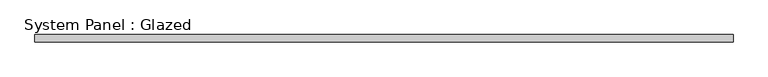
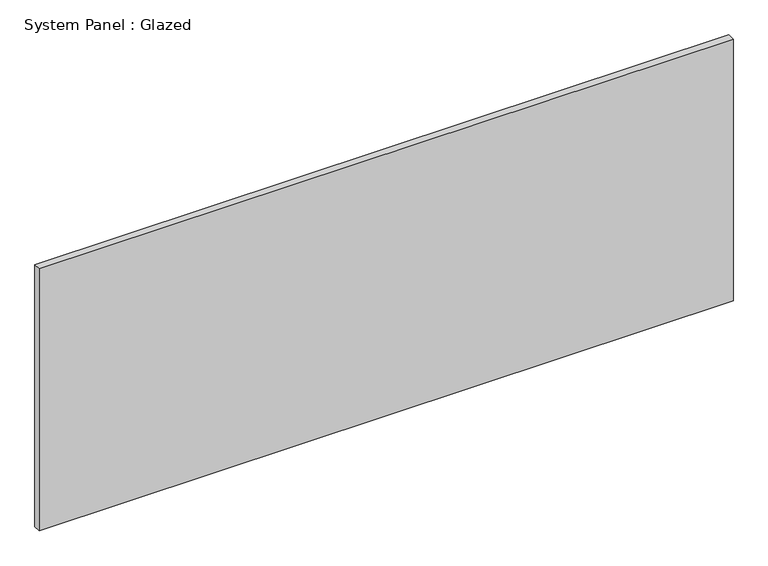
"""IFC4 building model written with IfcOpenShell, lengths in millimetres: plate geometry, System Panel : Glazed."""

from ifc_helpers import new_model, si_unit, origin, origin_with_axes, place, context, project, spatial, polyline, outline, extrude, source, transform, mapped, element, save


def system_panel_glazed_51b229ca(model_context):
    return source(origin(), model_context, "Body", "SweptSolid", [
        extrude(outline(polyline([(1199.1779362, 19.05), (-1199.1779362, 19.05), (-1199.1779362, 44.45), (1199.1779362, 44.45), (1199.1779362, 19.05)])), origin_with_axes(), (0.0, 0.0, 1.0), 956.7857817),
    ])


if __name__ == "__main__":
    model = new_model("IFC4")
    model_context = context("Model", 3, world=origin())
    ifc_project = project(units=[si_unit("LENGTHUNIT", "METRE", prefix="MILLI")], contexts=[model_context])
    site = spatial("IfcSite", under=ifc_project)
    building = spatial("IfcBuilding", under=site)
    placement = place(None, origin())
    system_panel_glazed_shape = system_panel_glazed_51b229ca(model_context)
    element("IfcPlate", 1, ObjectType="System Panel : Glazed", at=placement, inside=building, context=model_context, shape_type="MappedRepresentation", body=[
        mapped(system_panel_glazed_shape, transform((0.0, 0.0, 0.0), x_axis=(1.0, 0.0, 0.0), y_axis=(0.0, 1.0, 0.0), z_axis=(0.0, 0.0, 1.0))),
    ])
    save(model, "model.ifc")

# Revit data of these elements
# Type "System Panel : Glazed"
#   Construction Type Id = "GSP4R"
#   Analytic Construction = "1/8 in Pilkington single glazing"
#   Visual Light Transmittance = 0.9
#   Solar Heat Gain Coefficient = 0.86
#   Heat Transfer Coefficient (U) = 1.18115 BTU/(h·ft²·°F)
#   Define Thermal Properties by = 1
# Element 1 (IfcPlate, "System Panel : Glazed")
#   Materials on its faces: "Glass"
# Materials
#   "Glass": class "Glass", colour RGB 0 128 192, transparency 0.75, Description = "Soda Lime Glass", Cost = 0
